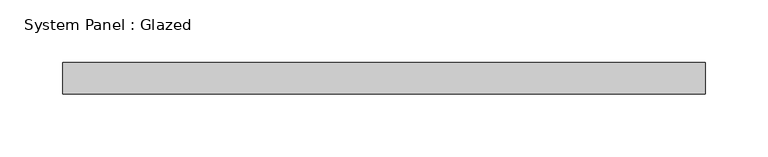
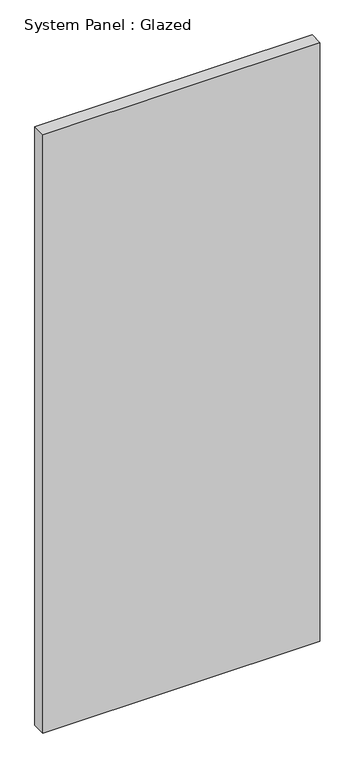
"""IFC4 building model written with IfcOpenShell, lengths in millimetres: plate geometry, System Panel : Glazed."""

from ifc_helpers import new_model, si_unit, origin, origin_with_axes, place, context, project, spatial, polyline, outline, extrude, source, transform, mapped, element, save


def system_panel_glazed_d098f70f(model_context):
    return source(origin(), model_context, "Body", "SweptSolid", [
        extrude(outline(polyline([(257.175, 19.05), (-257.175, 19.05), (-257.175, 44.45), (257.175, 44.45), (257.175, 19.05)])), origin_with_axes(), (0.0, 0.0, 1.0), 1174.6187331),
    ])


if __name__ == "__main__":
    model = new_model("IFC4")
    model_context = context("Model", 3, world=origin())
    ifc_project = project(units=[si_unit("LENGTHUNIT", "METRE", prefix="MILLI")], contexts=[model_context])
    site = spatial("IfcSite", under=ifc_project)
    building = spatial("IfcBuilding", under=site)
    placement = place(None, origin())
    system_panel_glazed_shape = system_panel_glazed_d098f70f(model_context)
    element("IfcPlate", 1, ObjectType="System Panel : Glazed", at=placement, inside=building, context=model_context, shape_type="MappedRepresentation", body=[
        mapped(system_panel_glazed_shape, transform((0.0, 0.0, 0.0), x_axis=(1.0, 0.0, 0.0), y_axis=(0.0, 1.0, 0.0), z_axis=(0.0, 0.0, 1.0))),
    ])
    save(model, "model.ifc")

# Revit data of these elements
# Type "System Panel : Glazed"
#   Construction Type Id = "GSP4R"
#   Analytic Construction = "1/8 in Pilkington single glazing"
#   Visual Light Transmittance = 0.9
#   Solar Heat Gain Coefficient = 0.86
#   Heat Transfer Coefficient (U) = 1.18115 BTU/(h·ft²·°F)
#   Define Thermal Properties by = 1
# Element 1 (IfcPlate, "System Panel : Glazed")
#   Materials on its faces: "Glass"
# Materials
#   "Glass": class "Glass", colour RGB 0 128 192, transparency 0.75, Description = "Soda Lime Glass", Cost = 0
